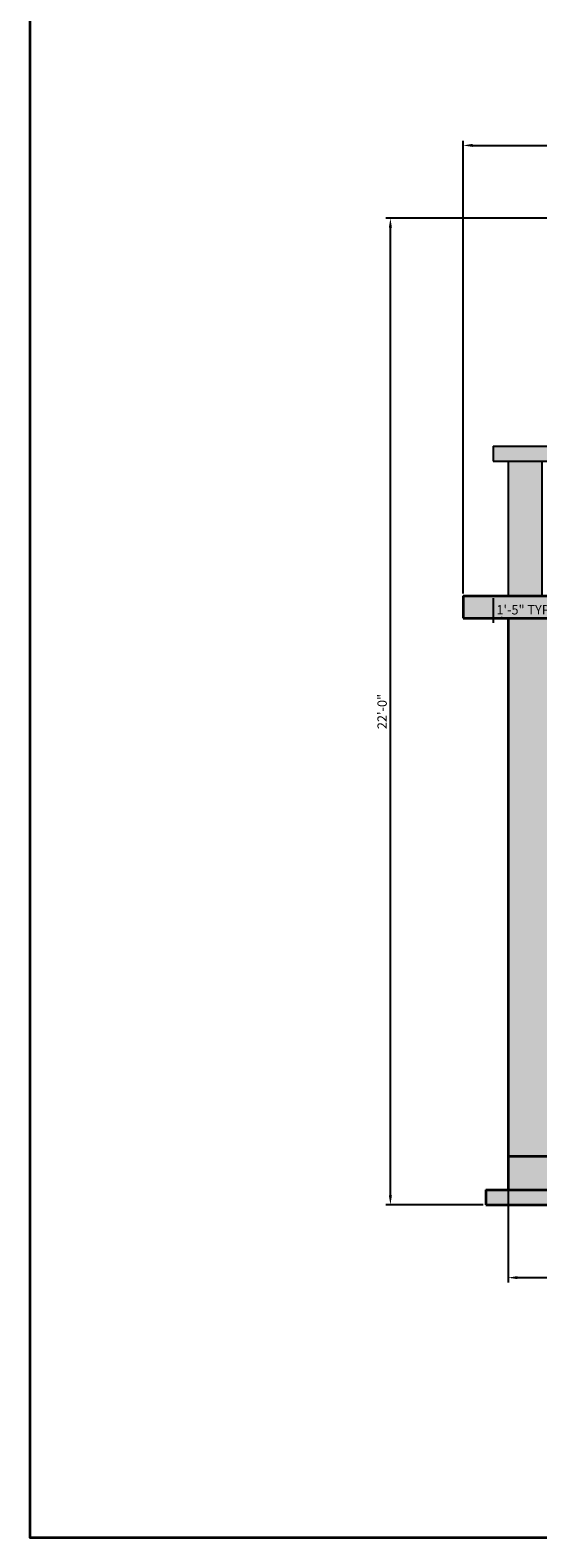
# Model space of a CAD drawing. Units: inches. Extents: x 2150 to 10686, y 1035 to 5077.
# Tile 5 of 12: x 6113 to 6249, y 4201 to 4605. Entities that reach past the tile are written whole.
import ezdxf

# ---------------------------------------------------------------- set-up
doc = ezdxf.new("R2010")
doc.units = ezdxf.units.IN
for name, color, linetype, lineweight in [('A-ANNO-DIMS', 2, 'Continuous', 18), ('A-ANNO-TTLB', 7, 'Continuous', 35), ('A-ELEV', 7, 'Continuous', 35), ('A-ELEV-BASE-PATT', 251, 'Continuous', 13), ('A-ELEV-METL-PATT', 252, 'Continuous', 13), ('A-ELEV-RAIL', 7, 'Continuous', 25)]:
    doc.layers.add(name, color=color, linetype=linetype, lineweight=lineweight)
for name, color, linetype, lineweight, true_color in [('A-ELEV-CONC-PATT', 253, 'Continuous', 13, 0xb2a88f), ('A-ELEV-PATT', 253, 'Continuous', 13, 0xa5adc8), ('A-ELEV-TRIM-PATT', 85, 'Continuous', 13, 0x58ba48)]:
    doc.layers.add(name, color=color, linetype=linetype, lineweight=lineweight, true_color=true_color)
doc.styles.get("Standard").update_dxf_attribs({"font": 'arial.ttf'})
doc.dimstyles.new('ISO-25', dxfattribs={"dimtxt": 2.5, "dimasz": 2.5, "dimexe": 1.25, "dimexo": 0.625, "dimtad": 1, "dimdec": 0, "dimlunit": 3, "dimtxsty": 'Standard', "dimcen": 2.5, "dimadec": 0, "dimazin": 0, "dimtfac": 1, "dimtdec": 0, "dimtmove": 0, "dimatfit": 3, "dimfxl": 1, "dimarcsym": 0})

# ---------------------------------------------------------------- blocks, each defined once
blk = doc.blocks.new('RAIL-POST-CAPPED')
for p, q in [((0, 40), (17, 40)), ((0, 40), (0, 36)), ((17, 40), (17, 36)), ((0, 36), (17, 36)), ((4, 36), (4, 0)), ((13, 36), (13, 0))]:
    blk.add_line(p, q)
blk = doc.blocks.new('*D65')
at = {"layer": 'A-ANNO-DIMS', "color": 0, "lineweight": -2, "transparency": 16777216}
for p, q in [((6236.61, 4452.86), (6236.61, 4446.23)), ((6253.61, 4452.86), (6253.61, 4446.23)), ((6239.11, 4447.48), (6251.11, 4447.48))]:
    blk.add_line(p, q, dxfattribs=at)
at = {"layer": 'A-ANNO-DIMS', "color": 0, "transparency": 16777216}
for points in [[(6239.11, 4447.9), (6239.11, 4447.07), (6236.61, 4447.48)], [(6251.11, 4447.9), (6251.11, 4447.07), (6253.61, 4447.48)]]:
    blk.add_solid(points, dxfattribs=at)
at = {"layer": 'Defpoints', "color": 0, "transparency": 16777216}
for p in [(6236.61, 4453.48), (6253.61, 4453.48), (6253.61, 4447.48)]:
    blk.add_point(p, dxfattribs=at)
at = {"layer": 'A-ANNO-DIMS', "color": 0, "transparency": 16777216, "insert": (6245.11, 4449.39), "char_height": 2.5, "attachment_point": 5}
blk.add_mtext('1\'-5" TYP.', dxfattribs=at)
blk = doc.blocks.new('*D126')
at = {"layer": 'A-ANNO-DIMS', "color": 0, "lineweight": -2, "transparency": 16777216}
for p, q in [((6228.61, 4454.11), (6228.61, 4575.23)), ((6231.11, 4573.98), (6490.11, 4573.98)), ((6492.61, 4454.11), (6492.61, 4575.23))]:
    blk.add_line(p, q, dxfattribs=at)
at = {"layer": 'A-ANNO-DIMS', "color": 0, "transparency": 16777216}
for points in [[(6231.11, 4574.4), (6231.11, 4573.57), (6228.61, 4573.98)], [(6490.11, 4574.4), (6490.11, 4573.57), (6492.61, 4573.98)]]:
    blk.add_solid(points, dxfattribs=at)
at = {"layer": 'Defpoints', "color": 0, "transparency": 16777216}
for p in [(6492.61, 4573.98), (6228.61, 4453.48), (6492.61, 4453.48)]:
    blk.add_point(p, dxfattribs=at)
at = {"layer": 'A-ANNO-DIMS', "color": 0, "transparency": 16777216, "insert": (6360.61, 4575.89), "char_height": 2.5, "attachment_point": 5}
blk.add_mtext('22\'-0"', dxfattribs=at)
blk = doc.blocks.new('*D127')
at = {"layer": 'A-ANNO-DIMS', "color": 0, "lineweight": -2, "transparency": 16777216}
for p, q in [((6336.98, 4554.48), (6207.86, 4554.48)), ((6209.11, 4292.98), (6209.11, 4551.98)), ((6233.98, 4290.48), (6207.86, 4290.48))]:
    blk.add_line(p, q, dxfattribs=at)
at = {"layer": 'A-ANNO-DIMS', "color": 0, "transparency": 16777216}
for points in [[(6208.69, 4551.98), (6209.52, 4551.98), (6209.11, 4554.48)], [(6208.69, 4292.98), (6209.52, 4292.98), (6209.11, 4290.48)]]:
    blk.add_solid(points, dxfattribs=at)
at = {"layer": 'Defpoints', "color": 0, "transparency": 16777216}
for p in [(6209.11, 4554.48), (6337.61, 4554.48), (6234.61, 4290.48)]:
    blk.add_point(p, dxfattribs=at)
at = {"layer": 'A-ANNO-DIMS', "color": 0, "transparency": 16777216, "insert": (6207.21, 4422.48), "char_height": 2.5, "attachment_point": 5, "rotation": 90}
blk.add_mtext('22\'-0"', dxfattribs=at)
blk = doc.blocks.new('*D134')
at = {"layer": 'A-ANNO-DIMS', "color": 0, "lineweight": -2, "transparency": 16777216}
for p, q in [((6240.61, 4302.86), (6240.61, 4269.73)), ((6318.61, 4302.86), (6318.61, 4269.73)), ((6243.11, 4270.98), (6316.11, 4270.98))]:
    blk.add_line(p, q, dxfattribs=at)
at = {"layer": 'A-ANNO-DIMS', "color": 0, "transparency": 16777216}
for points in [[(6243.11, 4271.4), (6243.11, 4270.57), (6240.61, 4270.98)], [(6316.11, 4271.4), (6316.11, 4270.57), (6318.61, 4270.98)]]:
    blk.add_solid(points, dxfattribs=at)
at = {"layer": 'Defpoints', "color": 0, "transparency": 16777216}
for p in [(6240.61, 4303.48), (6318.61, 4303.48), (6318.61, 4270.98)]:
    blk.add_point(p, dxfattribs=at)
at = {"layer": 'A-ANNO-DIMS', "color": 0, "transparency": 16777216, "insert": (6279.61, 4272.89), "char_height": 2.5, "attachment_point": 5}
blk.add_mtext('6\'-6"', dxfattribs=at)

msp = doc.modelspace()

# ---------------------------------------------------------------- hatches: boundary and pattern name
at = {"layer": 'A-ELEV-BASE-PATT'}
h = msp.add_hatch(color=256, dxfattribs=at)
h.dxf.hatch_style = 1
h.paths.add_polyline_path([(6480.63, 4303.48), (6240.61, 4303.48), (6240.61, 4294.48), (6480.63, 4294.48)])
h = msp.add_hatch(color=256, dxfattribs=at)
h.dxf.hatch_style = 1
h.paths.add_polyline_path([(6486.61, 4294.48), (6234.61, 4294.48), (6234.61, 4290.48), (6486.61, 4290.48)])
at = {"layer": 'A-ELEV-CONC-PATT'}
h = msp.add_hatch(dxfattribs=at)
h.set_pattern_fill('AR-CONC', color=256, scale=0.02)
h.paths.add_polyline_path([(6444.63, 4525.48), (6367.61, 4525.48), (6367.61, 4516.48), (6435.63, 4516.48), (6435.63, 4303.48), (6444.63, 4303.48)])
h.paths.add_polyline_path([(6367.61, 4453.48), (6228.61, 4453.48), (6228.61, 4447.48), (6367.61, 4447.48)])
h.paths.add_polyline_path([(6492.61, 4453.48), (6480.63, 4453.48), (6480.63, 4447.48), (6492.61, 4447.48)])
h.paths.add_polyline_path([(6492.61, 4554.48), (6337.61, 4554.48), (6337.61, 4549.48), (6492.61, 4549.48)])
at = {"layer": 'A-ELEV-METL-PATT'}
h = msp.add_hatch(color=256, dxfattribs=at)
h.dxf.hatch_style = 1
h.paths.add_polyline_path([(6253.61, 4493.48), (6236.61, 4493.48), (6236.61, 4489.48), (6253.61, 4489.48)])
h.paths.add_polyline_path([(6295.61, 4493.48), (6278.61, 4493.48), (6278.61, 4489.48), (6295.61, 4489.48)])
h.paths.add_polyline_path([(6337.61, 4493.48), (6320.61, 4493.48), (6320.61, 4489.48), (6337.61, 4489.48)])
at = {"layer": 'A-ELEV-PATT'}
h = msp.add_hatch(color=256, dxfattribs=at)
h.dxf.hatch_style = 1
h.paths.add_polyline_path([(6318.61, 4447.48), (6240.61, 4447.48), (6240.61, 4303.48), (6318.61, 4303.48)])
h.paths.add_polyline_path([(6294.61, 4387.48), (6294.61, 4369.48), (6264.61, 4369.48), (6264.61, 4387.48)], flags=16)
h.paths.add_polyline_path([(6291.61, 4384.48), (6291.61, 4372.48), (6267.61, 4372.48), (6267.61, 4384.48)], flags=0)
at = {"layer": 'A-ELEV-TRIM-PATT'}
h = msp.add_hatch(color=256, dxfattribs=at)
h.dxf.hatch_style = 1
h.paths.add_polyline_path([(6249.61, 4489.48), (6240.61, 4489.48), (6240.61, 4453.48), (6249.61, 4453.48)])
h.paths.add_polyline_path([(6291.61, 4489.48), (6282.61, 4489.48), (6282.61, 4453.48), (6291.61, 4453.48)])
h.paths.add_polyline_path([(6333.61, 4489.48), (6324.61, 4489.48), (6324.61, 4453.48), (6333.61, 4453.48)])

# ---------------------------------------------------------------- linework, layer by layer
at = {"layer": 'A-ANNO-TTLB'}
msp.add_lwpolyline([(6112.69, 5076.61), (7001.25, 5076.61), (7001.25, 4201.35), (6112.69, 4201.35)], close=True, dxfattribs=at)
at = {"layer": 'A-ELEV'}
for p, q in [((6228.61, 4453.48), (6367.61, 4453.48)), ((6228.61, 4453.48), (6228.61, 4447.48)), ((6228.61, 4447.48), (6367.61, 4447.48)), ((6240.61, 4447.48), (6240.61, 4294.48)), ((6240.61, 4303.48), (6480.61, 4303.48)), ((6234.61, 4294.48), (6486.61, 4294.48)), ((6234.61, 4294.48), (6234.61, 4290.48)), ((6234.61, 4290.48), (6486.61, 4290.48))]:
    msp.add_line(p, q, dxfattribs=at)

# ---------------------------------------------------------------- block references
at = {"layer": 'A-ELEV-RAIL'}
msp.add_blockref('RAIL-POST-CAPPED', (6236.61, 4453.48), dxfattribs=at)

# ---------------------------------------------------------------- dimensions: what is measured, and where the dimension line sits
at = {"layer": 'A-ANNO-DIMS'}
for base, p1, p2, picture, middle in [((6492.61, 4573.98), (6228.61, 4453.48), (6492.61, 4453.48), '*D126', (6360.61, 4575.89)), ((6318.61, 4270.98), (6240.61, 4303.48), (6318.61, 4303.48), '*D134', (6279.61, 4272.89))]:
    dim = msp.add_linear_dim(base=base, p1=p1, p2=p2, dimstyle='ISO-25', override={"dimdec": 1, "dimlfac": 1, "dimrnd": 0, "dimzin": 1, "dimdsep": 46, "dimlunit": 4, "dimfrac": 2}, dxfattribs=at)
    dim.commit()
    dim.dimension.update_dxf_attribs({"geometry": picture, "text_midpoint": middle})
dim = msp.add_linear_dim(base=(6209.11, 4554.48), p1=(6234.61, 4290.48), p2=(6337.61, 4554.48), angle=90, dimstyle='ISO-25', override={"dimdec": 1, "dimlfac": 1, "dimrnd": 0, "dimzin": 1, "dimdsep": 46, "dimlunit": 4, "dimfrac": 2}, dxfattribs=at)
dim.commit()
dim.dimension.update_dxf_attribs({"geometry": '*D127', "text_midpoint": (6207.21, 4422.48)})
dim = msp.add_linear_dim(base=(6253.61, 4447.48), p1=(6236.61, 4453.48), p2=(6253.61, 4453.48), text='<> TYP.', dimstyle='ISO-25', override={"dimdec": 1, "dimlfac": 1, "dimrnd": 0, "dimzin": 1, "dimdsep": 46, "dimlunit": 4, "dimfrac": 2}, dxfattribs=at)
dim.commit()
dim.dimension.update_dxf_attribs({"geometry": '*D65', "text_midpoint": (6245.11, 4449.39)})

doc.saveas('drawing.dxf')
